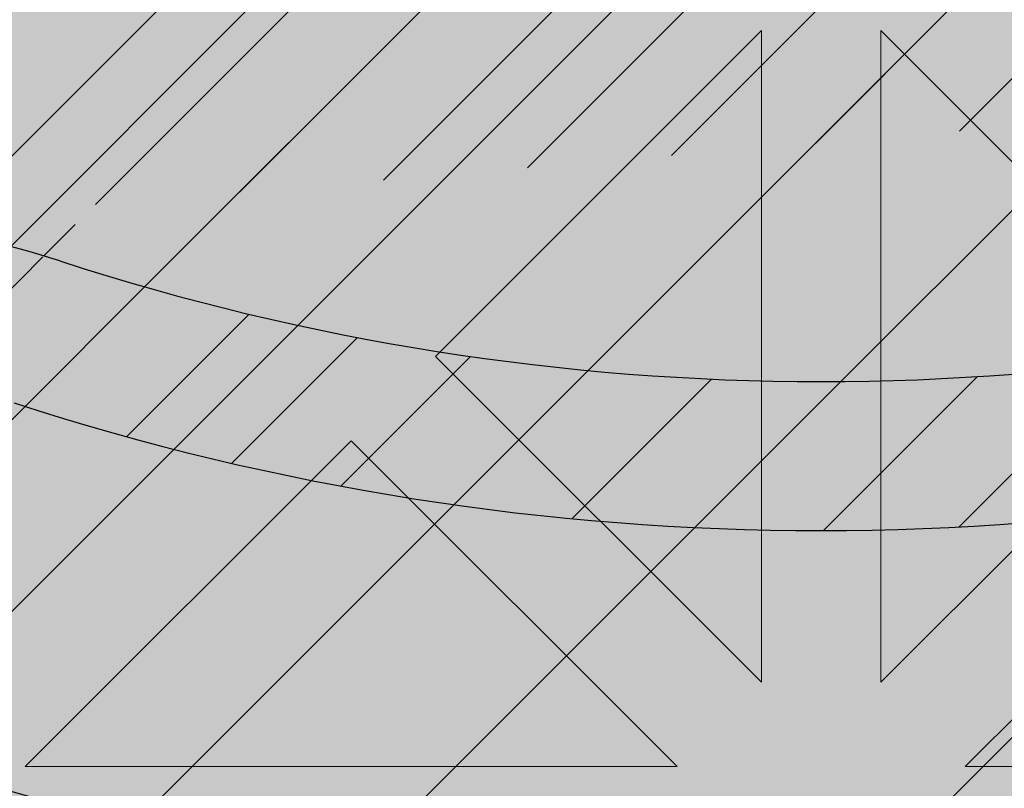
# Model space of a CAD drawing. Units: inches. Extents: x 844 to 2234, y 346 to 1084.
# Tile 10 of 93: x 1121.143 to 1123.249, y 688.619 to 690.263. Entities that reach past the tile are written whole.
import ezdxf

# ---------------------------------------------------------------- set-up
doc = ezdxf.new("R2010")
doc.units = ezdxf.units.IN
doc.header["$MEASUREMENT"] = 0
for name, color, linetype, lineweight in [('A-ANNO-DIMS', 2, 'Continuous', 18), ('furniture', 8, 'Continuous', 18), ('RA-AP-01$0$INT', 35, 'Continuous', 5)]:
    doc.layers.add(name, color=color, linetype=linetype, lineweight=lineweight)
doc.layers.add('RA-AP-01$0$FURN', color=3, linetype='Continuous')
doc.layers.add('RA-AP-01$0$WOOD', color=64, linetype='Continuous')
doc.styles.get("Standard").update_dxf_attribs({"font": 'arial.ttf'})
doc.dimstyles.get("Standard").update_dxf_attribs({"dimtxt": 6, "dimasz": 3, "dimexe": 0.18, "dimexo": 0.0625, "dimgap": 0.09, "dimtad": 0, "dimtih": 1, "dimtoh": 1, "dimdec": 1, "dimzin": 0, "dimdsep": 46, "dimlunit": 3, "dimtxsty": 'Standard', "dimblk": 'ARCHTICK', "dimcen": 0.09, "dimadec": 0, "dimazin": 0, "dimtfac": 1, "dimtdec": 1, "dimtofl": 0, "dimtmove": 0, "dimatfit": 3, "dimfxl": 1, "dimtolj": 1, "dimtzin": 0, "dimarcsym": 0})

# ---------------------------------------------------------------- blocks, each defined once
blk = doc.blocks.new('A$C18D01794')
at = {"layer": 'RA-AP-01$0$INT'}
h = blk.add_hatch(color=256, dxfattribs=at)
h.paths.add_polyline_path([(4.585917135068449, -6.356712009588271), (4.555206456959269, -6.35671200958746), (4.555206456959137, -6.387422687716308), (4.874495778835233, -6.706712009592356), (4.90520645695423, -6.676001331474049)])
h.paths.add_polyline_path([(5.255206456948813, -6.387422687716306), (5.255206456948682, -6.356712009605972), (5.224495778822613, -6.356712009605161), (4.905206456953498, -6.676001331474273), (4.935917135072151, -6.706712009592924)])
h.paths.add_polyline_path([(4.935917135072559, -6.706712009592068), (4.905206456953564, -6.737422687710376), (5.255206456951813, -7.087422687708613), (5.255206456951549, -7.026001331471008)])
h.paths.add_polyline_path([(4.555206456956399, -7.026001331471013), (4.555206456956134, -7.087422687708616), (4.905206456953821, -6.737422687710943), (4.874495778835166, -6.70671200959229)])
h = blk.add_hatch(color=256, dxfattribs=at)
h.paths.add_polyline_path([(4.585917135068448, -6.356712009588273), (4.614201406330596, -6.356712009589021), (4.668846067270487, -6.411356670531338), (4.723490728212344, -6.356712009591912), (4.771774999457151, -6.35671200959319), (4.826419660396886, -6.411356670535356), (4.862780050090322, -6.374996280843536), (4.844495778842715, -6.356712009595112), (4.862780050090411, -6.356712009595595), (4.905206456960182, -6.399138416468211), (4.947632863832445, -6.356712009597838), (4.965917135079675, -6.356712009598322), (4.947632863831759, -6.374996280845421), (4.983993253523576, -6.411356670538857), (5.038637914464627, -6.356712009600247), (5.08692218571208, -6.356712009601523), (5.141566846649976, -6.411356670541852), (5.196211507589851, -6.356712009604411), (5.224495778822615, -6.356712009605161), (4.905206456953975, -6.676001331473793)])
h.paths.add_polyline_path([(4.895206456956031, -6.637717060225675), (4.895206456958921, -6.528427738347902), (4.840561796018589, -6.583072399285802)], flags=16)
h.paths.add_polyline_path([(4.915206456955638, -6.637717060226121), (4.969851117895509, -6.583072399288678), (4.915206456957609, -6.528427738348344)], flags=16)
h.paths.add_polyline_path([(4.826419660395175, -6.568930263661755), (4.881064321335613, -6.514285602723745), (4.771774999456703, -6.514285602720857)], flags=16)
h.paths.add_polyline_path([(4.983993253519558, -6.568930263665262), (5.038637914460456, -6.514285602726792), (4.929348592581548, -6.514285602724816)], flags=16)
h.paths.add_polyline_path([(4.881064321336025, -6.494285602723742), (4.826419660397532, -6.439640941782821), (4.771774999457062, -6.494285602720859)], flags=16)
h.paths.add_polyline_path([(4.929348592582019, -6.494285602724817), (5.038637914460982, -6.494285602726792), (4.983993253522945, -6.439640941786327)], flags=16)
h.paths.add_polyline_path([(4.895206456960191, -6.480143467100443), (4.895206456962115, -6.407422687715913), (4.876922185715016, -6.389138416467584), (4.840561796021581, -6.425498806159401)], flags=16)
h.paths.add_polyline_path([(4.915206456958487, -6.480143467100889), (4.969851117899527, -6.425498806162279), (4.933490728206909, -6.389138416468043), (4.9152064569598, -6.40742268771434)], flags=16)
h.paths.add_polyline_path([(4.757632863832376, -6.480143467096812), (4.812277524772842, -6.425498806158772), (4.757632863834348, -6.370854145217844)], flags=16)
h.paths.add_polyline_path([(4.737632863832376, -6.480143467096286), (4.737632863834348, -6.370854145217375), (4.682988202893906, -6.425498806155385)], flags=16)
h.paths.add_polyline_path([(5.05278005008503, -6.480143467103376), (5.052780050087917, -6.370854145224413), (4.998135389146995, -6.425498806162908)], flags=16)
h.paths.add_polyline_path([(5.072780050085024, -6.480143467103744), (5.127424711025931, -6.42549880616527), (5.072780050087916, -6.370854145224832)], flags=16)
h.paths.add_polyline_path([(4.935917135072783, -6.706712009592292), (5.255206456948811, -6.387422687716309), (5.255206456948932, -6.415706958964177), (5.200561796010279, -6.470351619902839), (5.255206456949403, -6.524996280841948), (5.25520645694961, -6.5732805520894), (5.200561796009787, -6.627925213029239), (5.236922185702417, -6.664285602721864), (5.255206456949919, -6.646001331474357), (5.255206456949998, -6.664285602721898), (5.212780050078687, -6.706712009592262), (5.25520645695036, -6.749138416463932), (5.255206456950438, -6.767422687711313), (5.236922185702424, -6.749138416463297), (5.200561796009796, -6.785498806155928), (5.255206456950753, -6.840143467096874), (5.25520645695096, -6.888427738341682), (5.200561796010322, -6.943072399282328), (5.255206456951428, -6.997717060223427), (5.255206456951547, -7.026001331471006)])
h.paths.add_polyline_path([(5.042988202883395, -6.785498806155427), (5.097632863823085, -6.840143467095101), (5.097632863822622, -6.730854145216193)], flags=16)
h.paths.add_polyline_path([(5.028846067259663, -6.771356670531693), (5.083490728198774, -6.716712009592573), (4.974201406321001, -6.716712009593042)], flags=16)
h.paths.add_polyline_path([(5.117632863823087, -6.840143467095186), (5.172277524762331, -6.785498806155926), (5.11763286382262, -6.730854145216225)], flags=16)
h.paths.add_polyline_path([(5.08349072819877, -6.696712009593886), (5.028846067259652, -6.642067348654775), (4.974201406320998, -6.696712009593438)], flags=16)
h.paths.add_polyline_path([(5.131774999446817, -6.854285602718917), (5.186419660386065, -6.799640941779662), (5.241064321325782, -6.854285602719365)], flags=17)
h.paths.add_polyline_path([(5.131774999446228, -6.716712009592374), (5.186419660386065, -6.771356670532194), (5.222780050079488, -6.734996280838764), (5.204495778832781, -6.716712009592063)], flags=16)
h.paths.add_polyline_path([(5.097632863822613, -6.682569873970264), (5.097632863823061, -6.573280552091354), (5.042988202883383, -6.627925213031044)], flags=16)
h.paths.add_polyline_path([(5.131774999446899, -6.874285602718915), (5.241064321325809, -6.874285602719364), (5.186419660386591, -6.928930263658598)], flags=17)
h.paths.add_polyline_path([(5.131774999446226, -6.696712009594078), (5.204495778830767, -6.696712009594374), (5.22278005007868, -6.67842773834687), (5.186419660386049, -6.642067348654249)], flags=16)
h.paths.add_polyline_path([(5.11763286382262, -6.682569873970225), (5.17227752476232, -6.627925213030515), (5.117632863823064, -6.573280552091267)], flags=16)
h.paths.add_polyline_path([(5.186419660386069, -6.613783077405491), (5.241064321325754, -6.559138416465795), (5.131774999446791, -6.559138416466263)], flags=16)
h.paths.add_polyline_path([(5.131774999446872, -6.539138416466263), (5.24106432132578, -6.539138416465794), (5.186419660386554, -6.484493755526573)], flags=16)
h.paths.add_polyline_path([(5.255206456951811, -7.08742268770861), (5.255206456951895, -7.106712009588038), (4.555206456956052, -7.106712009588038), (4.555206456956136, -7.087422687708617), (4.905206456953973, -6.737422687710788)])
h.paths.add_polyline_path([(4.983993253513404, -6.8444937555241), (4.92934859257295, -6.899138416462108), (5.03863791445186, -6.899138416465014)], flags=16)
h.paths.add_polyline_path([(4.969851117889988, -6.83035161990006), (4.915206456952556, -6.775706958960171), (4.915206456949648, -6.884996280837944)], flags=16)
h.paths.add_polyline_path([(4.929348592572535, -6.919138416462105), (4.983993253511019, -6.973783077403037), (5.038637914451496, -6.919138416465012)], flags=16)
h.paths.add_polyline_path([(5.052780050074912, -6.93328055208906), (4.998135389134438, -6.987925213027088), (5.052780050072919, -7.042569873968025)], flags=16)
h.paths.add_polyline_path([(5.07278005007491, -6.933280552089588), (5.072780050072918, -7.042569873968497), (5.127424711013374, -6.987925213030498)], flags=16)
h.paths.add_polyline_path([(4.89520645695295, -6.775706958959721), (4.840561796013067, -6.830351619897157), (4.895206456950961, -6.884996280837494)], flags=16)
h.paths.add_polyline_path([(4.915206456948365, -6.933280552085403), (4.915206456946434, -7.006001331471951), (4.933490728192729, -7.024285602719066), (4.969851117886972, -6.987925213026453)], flags=16)
h.paths.add_polyline_path([(4.881064321327021, -6.899138416461022), (4.82641966038902, -6.84449375552057), (4.771774999448108, -6.899138416459029)], flags=16)
h.paths.add_polyline_path([(4.895206456950073, -6.933280552084951), (4.840561796009022, -6.987925213023558), (4.876922185700835, -7.024285602716997), (4.895206456948749, -7.006001331469487)], flags=16)
h.paths.add_polyline_path([(4.983993253510392, -7.0020673486505), (4.947632863816944, -7.038427738342319), (4.965917135064043, -7.05671200959023), (5.038637914448995, -7.056712009591555)], flags=16)
h.paths.add_polyline_path([(4.881064321326543, -6.91913841646102), (4.771774999447578, -6.919138416459031), (4.826419660385607, -6.973783077399508)], flags=16)
h.paths.add_polyline_path([(4.905206456946447, -7.014285602717636), (4.862780050074785, -7.056712009588352), (4.947632863816685, -7.056712009589775)], flags=16)
h.paths.add_polyline_path([(5.14156684663679, -7.002067348654549), (5.086922185696452, -7.056712009592438), (5.196211507574223, -7.056712009594425)], flags=16)
h.paths.add_polyline_path([(4.8264196603837, -7.002067348646972), (4.771774999442643, -7.056712009585575), (4.8444957788276, -7.056712009587508), (4.862780050075511, -7.038427738340416)], flags=16)
h.paths.add_polyline_path([(4.812277524760289, -6.98792521302292), (4.757632863822258, -6.933280552082447), (4.757632863819352, -7.042569873961408)], flags=16)
h.paths.add_polyline_path([(4.73763286382226, -6.933280552082079), (4.682988202881349, -6.987925213020536), (4.737632863819352, -7.04256987396099)], flags=16)
h.paths.add_polyline_path([(4.723490728195188, -7.056712009584289), (4.668846067257299, -7.002067348643949), (4.614201406317417, -7.056712009581383)], flags=16)
h.paths.add_polyline_path([(4.597632863829262, -6.706712009592262), (4.555206456957951, -6.664285602721896), (4.555206456958029, -6.646001331474357), (4.573490728205535, -6.664285602721864), (4.609851117898167, -6.627925213029238), (4.555206456958338, -6.573280552089402), (4.555206456958546, -6.524996280841952), (4.60985111789767, -6.470351619902839), (4.555206456959015, -6.415706958964177), (4.555206456959138, -6.387422687716309), (4.874495778835167, -6.70671200959229), (4.5552064569564, -7.026001331471015), (4.555206456956523, -6.997717060223433), (4.609851117897629, -6.94307239928233), (4.555206456956988, -6.888427738341681), (4.555206456957198, -6.840143467096881), (4.609851117898153, -6.78549880615593), (4.573490728205528, -6.749138416463297), (4.555206456957507, -6.76742268771132), (4.555206456957585, -6.749138416463933)])
h.paths.add_polyline_path([(4.712780050085332, -6.730854145216195), (4.712780050084863, -6.840143467095105), (4.767424711024555, -6.785498806155427)], flags=16)
h.paths.add_polyline_path([(4.726922185709173, -6.716712009592573), (4.781566846648288, -6.771356670531693), (4.836211507586949, -6.716712009593043)], flags=16)
h.paths.add_polyline_path([(4.692780050085327, -6.730854145216225), (4.638135389145619, -6.785498806155928), (4.692780050084865, -6.840143467095185)], flags=16)
h.paths.add_polyline_path([(4.726922185709182, -6.696712009593886), (4.836211507586949, -6.696712009593436), (4.7815668466483, -6.642067348654773)], flags=16)
h.paths.add_polyline_path([(4.678637914461726, -6.71671200959237), (4.605917135075169, -6.716712009592063), (4.587632863828464, -6.734996280838766), (4.623993253521887, -6.771356670532195)], flags=16)
h.paths.add_polyline_path([(4.712780050085336, -6.68256987397026), (4.767424711024568, -6.627925213031042), (4.71278005008489, -6.573280552091352)], flags=16)
h.paths.add_polyline_path([(4.678637914461726, -6.696712009594076), (4.623993253521899, -6.642067348654247), (4.587632863829271, -6.67842773834687), (4.605917135077185, -6.696712009594376)], flags=16)
h.paths.add_polyline_path([(4.692780050085336, -6.682569873970228), (4.692780050084889, -6.573280552091267), (4.638135389145632, -6.627925213030515)], flags=16)
h.paths.add_polyline_path([(4.623993253521885, -6.799640941779662), (4.678637914461131, -6.854285602718915), (4.56934859258217, -6.854285602719365)], flags=17)
h.paths.add_polyline_path([(4.623993253521901, -6.613783077405509), (4.678637914461158, -6.559138416466263), (4.569348592582195, -6.559138416465795)], flags=16)
h.paths.add_polyline_path([(4.678637914461051, -6.874285602718915), (4.623993253521361, -6.928930263658598), (4.569348592582143, -6.874285602719364)], flags=17)
h.paths.add_polyline_path([(4.678637914461076, -6.539138416466263), (4.623993253521399, -6.484493755526573), (4.569348592582167, -6.539138416465796)], flags=16)
h = blk.add_hatch(color=256, dxfattribs=at)
h.paths.add_polyline_path([(4.969851117891331, -6.583072399286455), (4.915206456952669, -6.63771706022511), (4.915206456952222, -6.528427738347337)])
h.paths.add_polyline_path([(4.895206456953064, -6.637717060225108), (4.840561796014413, -6.583072399286448), (4.895206456953533, -6.528427738347335)])
h.paths.add_polyline_path([(4.826419660390684, -6.568930263662714), (4.771774999451003, -6.514285602723024), (4.881064321329913, -6.514285602723489)])
h.paths.add_polyline_path([(4.881064321329884, -6.494285602723492), (4.771774999450921, -6.494285602723024), (4.82641966039018, -6.439640941783778)])
h.paths.add_polyline_path([(4.895206456953734, -6.48014346709988), (4.840561796013912, -6.425498806160046), (4.876922185707337, -6.389138416466622), (4.895206456954043, -6.40742268771333)])
h.paths.add_polyline_path([(4.862780050082808, -6.374996280843689), (4.826419660390178, -6.411356670536314), (4.771774999450351, -6.356712009596481), (4.844495778835303, -6.356712009596181)])
h.paths.add_polyline_path([(4.812277524766446, -6.425498806160041), (4.757632863827191, -6.480143467099289), (4.757632863826741, -6.370854145220329)])
h.paths.add_polyline_path([(4.737632863827191, -6.480143467099214), (4.682988202887508, -6.425498806159518), (4.737632863826743, -6.370854145220299)])
h.paths.add_polyline_path([(4.668846067263777, -6.41135667053579), (4.614201406325123, -6.356712009597128), (4.723490728202894, -6.356712009596675)])
h.paths.add_polyline_path([(4.905206456953846, -6.399138416467422), (4.862780050082654, -6.356712009596229), (4.947632863824561, -6.356712009595756)])
h.paths.add_polyline_path([(4.915206456952028, -6.480143467099882), (4.91520645695173, -6.407422687715346), (4.933490728199234, -6.389138416467428), (4.96985111789186, -6.425498806160055)])
h.paths.add_polyline_path([(5.038637914454841, -6.494285602723048), (4.929348592575874, -6.494285602723497), (4.983993253515593, -6.439640941783787)])
h.paths.add_polyline_path([(4.983993253515065, -6.568930263662725), (4.929348592575849, -6.514285602723495), (5.038637914454755, -6.514285602723045)])
h.paths.add_polyline_path([(5.052780050079843, -6.480143467099317), (4.998135389140595, -6.425498806160058), (5.052780050080309, -6.370854145220356)])
h.paths.add_polyline_path([(4.983993253516868, -6.411356670536324), (4.947632863824241, -6.374996280843694), (4.965917135071747, -6.356712009596188), (5.038637914456701, -6.356712009596504)])
h.paths.add_polyline_path([(5.127424711019533, -6.425498806159557), (5.072780050079843, -6.480143467099239), (5.07278005008031, -6.370854145220326)])
h.paths.add_polyline_path([(5.141566846643269, -6.411356670535829), (5.086922185704154, -6.356712009596707), (5.196211507581929, -6.356712009597176)])
for p, q in [((4.905206456953975, -6.676001331473793), (4.585917135071132, -6.356712009590955)), ((4.874495778835167, -6.70671200959229), (4.555206456959136, -6.387422687716307)), ((4.771774999456703, -6.514285602720857), (4.881064321335613, -6.514285602723743)), ((4.826419660395171, -6.568930263661755), (4.771774999456703, -6.514285602720857)), ((4.881064321335613, -6.514285602723743), (4.826419660395173, -6.568930263661757)), ((4.929348592581546, -6.514285602724816), (4.983993253519556, -6.568930263665262)), ((5.038637914460456, -6.514285602726792), (4.929348592581546, -6.514285602724816)), ((4.895206456958917, -6.528427738347906), (4.840561796018589, -6.583072399285802)), ((4.895206456958921, -6.528427738347904), (4.895206456956031, -6.637717060225675)), ((4.915206456957613, -6.52842773834835), (4.969851117895507, -6.583072399288678)), ((4.915206456957609, -6.528427738348348), (4.915206456955636, -6.637717060226119)), ((4.895206456956031, -6.637717060225675), (4.840561796018589, -6.583072399285802)), ((4.915206456955636, -6.637717060226119), (4.969851117895507, -6.583072399288678))]:
    blk.add_line(p, q, dxfattribs=at)
blk = doc.blocks.new('A$C32926AE1')
at = {"layer": 'RA-AP-01$0$FURN'}
h = blk.add_hatch(dxfattribs=at)
h.set_pattern_fill('ANSI31', color=256, scale=0.1, style=0)
h.set_pattern_definition([(45, (0, 0), (-0.0088388347648318, 0.0088388347648318), [])])
edge = h.paths.add_edge_path(flags=16)
edge.add_arc((4.904771284329206, 4.246793130718756), 0.2603971832811541, 75.22398030683196, 104.7760196931204)
edge.add_arc((4.904771284329206, 4.246793130718756), 0.2603971832811541, 75.223980306832, 104.77601969312039, ccw=False)
edge = h.paths.add_edge_path(flags=16)
edge.add_arc((4.904771284329206, 4.067062675376612), 0.2603971832811541, 255.2239803068796, 284.776019693168)
edge.add_arc((4.904771284329206, 4.067062675376612), 0.2603971832811541, 255.22398030687958, 284.77601969316805, ccw=False)
edge = h.paths.add_edge_path(flags=0)
edge.add_arc((4.904771284329206, 4.067062675376612), 0.2603971832811541, 255.2239803068796, 284.776019693168)
edge.add_arc((4.904771284329206, 4.067062675376612), 0.2603971832811541, 255.22398030687958, 284.77601969316805, ccw=False)
edge = h.paths.add_edge_path(flags=0)
edge.add_arc((4.904771284329206, 4.067062675376612), 0.2603971832811541, 255.2239803068796, 284.776019693168)
edge.add_arc((4.904771284329206, 4.067062675376612), 0.2603971832811541, 255.22398030687958, 284.77601969316805, ccw=False)
edge = h.paths.add_edge_path()
edge.add_arc((4.604388392048174, 4.588829985554312), 0.1599999999999918, 342.3781640246255, 354.4317409793762)
edge.add_arc((5.090145208887507, 4.43216705527679), 0.3503971832811637, 162.0091218307731, 180.3186872093483)
edge.add_arc((5.205154176610243, 4.588829985554953), 0.1599999999999917, 185.5682590208461, 197.6218359767349)
edge.add_arc((4.904771284329229, 4.246793130718735), 0.3503971832811761, 72.00912183053516, 107.9908781690354)
edge.add_arc((9.535952835716557, 4.28682295566602), 4.798342501046485, 178.2875002453811, 181.5576802719453)
edge.add_arc((4.719397359771122, 4.43216705527679), 0.3503971832811637, 359.6813127906516, 377.9908781692269)
edge.add_arc((9.535967292294904, 4.286822350292874), 4.778371420254705, 178.2965938931842, 181.5667745797229)
edge.add_arc((4.719397359771122, 4.43216705527679), 0.3303971832811637, 359.6813127906516, 377.9908781692269)
edge.add_arc((0.2735752763637294, 4.286822350292874), 4.7783714202547, 358.4332254202771, 361.7034061068158)
edge.add_arc((5.061434214606998, 4.732549947558029), 0.1600000000000254, 252.3781640250584, 264.4317409792362)
edge.add_arc((4.748108354051257, 4.732549947558012), 0.1600000000000541, 275.5682590208426, 287.6218359759532)
edge.add_arc((4.604388392048115, 4.588829985554317), 0.1800000000000505, 342.3567572500182, 349.3735009646207)
edge.add_arc((5.205154176610254, 4.588829985554976), 0.1800000000000069, 190.6264990356027, 197.6432427513933)
edge.add_arc((5.061434214607106, 4.732549947558013), 0.1800000000000424, 252.3567572496606, 259.3735009644582)
edge.add_arc((4.904771284329208, 4.246793130718737), 0.3303971832811676, 71.99844483668534, 108.0015551637021)
edge.add_arc((4.748108354051414, 4.732549947558045), 0.1800000000000547, 280.6264990355479, 287.6432427495938)
edge.add_arc((5.090145208887514, 4.432167055276789), 0.2803971832811691, 162.8706300666893, 180.816523289902)
edge.add_arc((4.719397359771136, 4.432167055276689), 0.2803971832811534, 359.183476710103, 377.1293699333214)
edge.add_arc((4.904771284329222, 4.246793130718737), 0.2803971832811769, 72.87063006672916, 107.1293699332334)
edge.add_arc((5.090145208887522, 4.432167055276788), 0.2603971832811776, 165.2239803068007, 180.9953123810312)
edge.add_arc((4.719397359771141, 4.432167055276699), 0.2603971832811458, 359.0046876189768, 374.7760196932087)
edge.add_arc((5.090145208887507, 4.43216705527679), 0.3303971832811637, 162.0091218307731, 180.3186872093483)
edge.add_arc((9.53595427642584, 4.285015535491528), 4.728345371032053, 178.265043920078, 181.5679956281801)
edge.add_arc((0.2735882922327999, 4.285015535491582), 4.728345371032045, 358.4320043718193, 361.7349560799204)
edge.add_arc((9.535953591267507, 4.284458026472751), 4.708343996644348, 178.2573054306777, 181.5704995759608)
edge.add_arc((0.273588977391114, 4.284458026472785), 4.708343996644358, 358.4295004240388, 361.7426945693213)
edge.add_arc((0.2735889773911131, 4.029397779622582), 4.708343996644359, 358.2573054306787, 361.5704995759613)
edge.add_arc((9.535953591267518, 4.029397779622618), 4.708343996644359, 178.4295004240391, 181.7426945693223)
edge.add_arc((0.2735882922327901, 4.028840270603786), 4.728345371032054, 358.2650439200796, 361.5679956281808)
edge.add_arc((9.53595427642584, 4.028840270603841), 4.728345371032054, 178.4320043718199, 181.7349560799219)
edge.add_arc((0.2735752763637302, 4.027033455802493), 4.778371420254699, 358.2965938931842, 361.5667745797229)
edge.add_arc((4.719397359771122, 3.881688750818578), 0.3303971832811637, 342.0091218307731, 360.3186872093484)
edge.add_arc((5.090145208887507, 3.881688750818578), 0.3303971832811637, 179.6813127906516, 197.9908781692269)
edge.add_arc((9.535967292294904, 4.027033455802493), 4.778371420254705, 178.433225420277, 181.7034061068158)
edge.add_arc((4.719397359771122, 3.881688750818578), 0.3503971832811637, 342.0091218307731, 360.3186872093484)
edge.add_arc((9.53595283571655, 4.027032850429349), 4.79834250104648, 178.4423197280546, 181.7124997546188)
edge.add_arc((4.719397359771141, 3.881688750818669), 0.2603971832811458, 345.2239803067913, 360.9953123810232)
edge.add_arc((5.090145208887522, 3.88168875081858), 0.2603971832811776, 179.0046876189687, 194.7760196931993)
edge.add_arc((4.904771284329222, 4.067062675376631), 0.2803971832811769, 252.8706300667665, 287.1293699332708)
edge.add_arc((4.719397359771136, 3.881688750818678), 0.2803971832811534, 342.8706300666787, 360.8165232898969)
edge.add_arc((5.090145208887514, 3.881688750818579), 0.2803971832811691, 179.183476710098, 197.1293699333106)
edge.add_arc((4.748108354051414, 3.581305858537323), 0.1800000000000547, 72.3567572504062, 79.37350096445199)
edge.add_arc((4.904771284329208, 4.067062675376631), 0.3303971832811676, 251.9984448362979, 288.0015551633146)
edge.add_arc((5.061434214607106, 3.581305858537355), 0.1800000000000424, 100.6264990355418, 107.6432427503394)
edge.add_arc((5.205154176610254, 3.725025820540392), 0.1800000000000069, 162.3567572486066, 169.3735009643972)
edge.add_arc((4.604388392048115, 3.725025820541051), 0.1800000000000505, 10.62649903537925, 17.64324274998182)
edge.add_arc((4.748108354051257, 3.581305858537356), 0.1600000000000541, 72.37816402404681, 84.43174097915735)
edge.add_arc((4.904771284329229, 4.067062675376632), 0.3503971832811761, 252.0091218309645, 287.9908781694648)
edge.add_arc((5.061434214606998, 3.581305858537339), 0.1600000000000254, 95.56825902076373, 107.6218359749416)
edge.add_arc((5.205154176610243, 3.725025820540414), 0.1599999999999917, 162.3781640232651, 174.4317409791539)
edge.add_arc((5.090145208887507, 3.881688750818578), 0.3503971832811637, 179.6813127906516, 197.9908781692269)
edge.add_arc((4.604388392048174, 3.725025820541056), 0.1599999999999918, 5.568259020623824, 17.62183597537444)
edge.add_arc((0.2735897329420762, 4.28682295566602), 4.798342501046482, 358.4423197280547, 361.7124997546188)
edge.add_arc((0.2735897329420691, 4.027032850429348), 4.798342501046489, 358.2875002453812, 361.5576802719453)
at = {"layer": 'RA-AP-01$0$WOOD'}
h = blk.add_hatch(color=256, dxfattribs=at)
h.dxf.hatch_style = 1
h.paths.add_polyline_path([(5.157430609644524, 4.573483066760929, -0.1009492694046607), (5.155401577623758, 4.593365984175333, -0.1842662638101597), (5.172249623284174, 4.638795604568598, 0.2056608120311276), (5.179560981299304, 4.661316324430096, 0.3614336704623542), (5.134352340494423, 4.706524965234944, 0.2056608120311297), (5.111831620632933, 4.699213607219793, -0.1842662638101113), (5.066402000239693, 4.682365561559342, -0.1055311479399994), (5.045656153913092, 4.68467289944697, 0.1567636581983829), (4.763886414745334, 4.684672899446966, -0.1055311479399895), (4.743140568418733, 4.68236556155934, -0.1842662638100833), (4.6977109480255, 4.69921360721979, 0.2056608120302612), (4.675190228164109, 4.706524965234949, 0.3614336704708441), (4.629981587358889, 4.66131632442871, 0.2056608120245944), (4.637292945374126, 4.638795604567974, -0.1842662638101024), (4.654140991034615, 4.59336598417475, -0.1009492694055169), (4.652111959013835, 4.573483066760181, 0.021410119221476), (4.629748025606143, 4.156712009541676, 0.0214101192214795), (4.652111959013809, 3.739940952323101, -0.1009492694059586), (4.654140991034615, 3.720058034908448, -0.1842662638100975), (4.637292945374126, 3.674628414515226, 0.2056608120245705), (4.629981587358889, 3.652107694654492, 0.3614336704708879), (4.675190228164113, 3.606899053848249, 0.2056608120302384), (4.697710948025501, 3.614210411863408, -0.1842662638100995), (4.743140568418738, 3.63105845752386, -0.1055311479402541), (4.763886414745388, 3.628751119636215, 0.1567636581983776), (5.045656153913137, 3.628751119636244, -0.1055311479397538), (5.066402000239692, 3.631058457523857, -0.1842662638101067), (5.111831620632931, 3.614210411863407, 0.2056608120310924), (5.134352340494417, 3.606899053848256, 0.3614336704624001), (5.179560981299307, 3.652107694653103, 0.2056608120311314), (5.172249623284175, 3.6746284145146, -0.1842662638101402), (5.155401577623758, 3.72005803490786, -0.1009492694051366), (5.15743060964455, 3.739940952322354, 0.0214101192215073), (5.179794543052287, 4.156712009541468, 0.0214101192215252)])
h.paths.add_polyline_path([(4.639748609479751, 4.156712009541513, 0.0213537860821624), (4.661970494867118, 3.741887061152232, -0.094075836301374), (4.664143710413708, 3.7196126951003, -0.1824818158568985), (4.644813765429836, 3.668037719127816, 0.2056608120245319), (4.639939526753007, 3.653023905887301, 0.3614336704710246), (4.676106439397173, 3.616856993242342, 0.2056608120302234), (4.691120252638095, 3.621731231919122, -0.1824818158602558), (4.742695228611606, 3.641061176902986, -0.1029891339458722), (4.766991894714349, 3.638256818950944, 0.156709409989566), (5.042550673941472, 3.638256818950105, -0.102989133958497), (5.066847340047078, 3.641061176902949, -0.1824818158594995), (5.118422316020358, 3.621731231919103, 0.2056608120311416), (5.133436129261316, 3.616856993242346, 0.3614336704621468), (5.169603041905217, 3.653023905886178, 0.2056608120310986), (5.164728803228477, 3.668037719127177, -0.1824818158565612), (5.145398858244737, 3.719612695099578, -0.0940758363009313), (5.147572073791232, 3.741887061151398, 0.0213537860822023), (5.169793959178681, 4.156712009541451, 0.0213537860822226), (5.147572073791203, 4.571536957931898, -0.0940758363005034), (5.145398858244737, 4.59381132398362, -0.1824818158565587), (5.164728803228476, 4.645386299956021, 0.2056608120311045), (5.169603041905216, 4.66040011319702, 0.3614336704621845), (5.133436129261313, 4.696567025840856, 0.2056608120310773), (5.118422316020359, 4.691692787164098, -0.182481815859508), (5.066847340047078, 4.67236284218025, -0.1029891339584606), (5.04255067394148, 4.675167200133092, 0.156709409989566), (4.766991894714357, 4.675167200132257, -0.1029891339458842), (4.742695228611611, 4.672362842180213, -0.1824818158602725), (4.691120252638095, 4.691692787164077, 0.2056608120302152), (4.676106439397174, 4.696567025840858, 0.3614336704710363), (4.639939526753005, 4.660400113195899, 0.2056608120245495), (4.644813765429837, 4.645386299955384, -0.1824818158568934), (4.664143710413708, 4.593811323982902, -0.0940758363009187), (4.661970494867149, 4.571536957931074, 0.021353786082177)], flags=16)
h.paths.add_polyline_path([(5.129794543052235, 4.432167055276933, -0.0141661062790638), (5.130152669293814, 4.156927903047693, -0.0141661062790647), (5.129794543052234, 3.881688750818433, -0.0785247771143638), (5.10979738006795, 3.755143611847103, 0.0945969212073497), (5.105408519571111, 3.717898134952927, 0.1043170707844957), (5.116074640131521, 3.670385395016088, 0.1043170707864965), (5.068561900193738, 3.681051515576561, 0.09459692119553), (5.031316423304057, 3.676662655080835, -0.1580239521427272), (4.778226145355827, 3.676662655080367, 0.0945969211986668), (4.740980668464973, 3.681051515576592, 0.1043170707882822), (4.693467928526415, 3.670385395015844, 0.1043170707867916), (4.704134049087309, 3.717898134953662, 0.0945969211972894), (4.69974518859162, 3.755143611844042, -0.0785247771163196), (4.679748025606343, 3.881688750818406, -0.0141661062790663), (4.679389899364763, 4.156927903047693, -0.0141661062790672), (4.679748025606343, 4.432167055276998, -0.0785247771163064), (4.699745188591625, 4.55871219425134, 0.094596921197333), (4.704134049087308, 4.595957671141738, 0.1043170707867205), (4.693467928526416, 4.643470411079523, 0.1043170707882628), (4.740980668464965, 4.632804290518776, 0.0945969211988114), (4.778226145355874, 4.637193151015016, -0.158023952142669), (5.031316423304015, 4.637193151014546, 0.0945969211956361), (5.068561900193736, 4.632804290518806, 0.1043170707864979), (5.11607464013152, 4.643470411079278, 0.1043170707844617), (5.105408519571112, 4.595957671142455, 0.0945969212074597), (5.109797380067959, 4.558712194248236, -0.0785247771143467)], flags=0)
h.paths.add_polyline_path([(5.119794532311105, 4.432259799204851, -0.0142000800617244), (5.120156169157484, 4.156927903047701, -0.0142000800617277), (5.119794532311105, 3.881596006890482, -0.0784894509520253), (5.100273383573699, 3.758192358677797, 0.0940138827242913), (5.095413455884425, 3.717477693979438, 0.0606271852308753), (5.099615656341024, 3.686844378806616, 0.0606271852322524), (5.068982341167493, 3.691046579263239, 0.0940138827010453), (5.028267676478798, 3.686186651576848, -0.1580706864508061), (4.781274892180912, 3.686186651576435, 0.0940138827026903), (4.740560227491556, 3.691046579263279, 0.0606271852339895), (4.709926912317155, 3.686844378806508, 0.0606271852329405), (4.714129112773991, 3.717477693980356, 0.094013882701304), (4.709269185087677, 3.758192358669163, -0.0784894509577193), (4.689748036347473, 3.881596006890469, -0.014200080061729), (4.689386399501094, 4.156927903047709, -0.0142000800617217), (4.689748036347473, 4.432259799204808, -0.078489450957724), (4.709269185087651, 4.555663447426125, 0.0940138827014585), (4.714129112773992, 4.596378112114996, 0.0606271852329731), (4.709926912317154, 4.62701142728886, 0.0606271852340196), (4.74056022749157, 4.622809226832087, 0.0940138827024997), (4.781274892180847, 4.627669154518912, -0.1580706864508359), (5.028267676478777, 4.627669154518526, 0.0940138827010946), (5.068982341167492, 4.622809226832129, 0.060627185232254), (5.099615656341024, 4.627011427288751, 0.0606271852308727), (5.095413455884425, 4.59637811211593, 0.0940138827241088), (5.100273383573675, 4.555663447417647, -0.0784894509520978)], flags=0)
h.paths.add_polyline_path([(5.06978912287499, 4.430218106756144, -0.014241683694547), (5.070173729147532, 4.156927903047672, -0.0142416836945458), (5.06978912287499, 3.883637699339223, -0.0800609523125196), (5.052662118612511, 3.773463122773442, 0.0526421978001116), (5.04590916754064, 3.740550867606997, 0.0526421977992423), (5.012996912374707, 3.73379791653534, -0.1583028414718258), (4.796545656286308, 3.73379791653451, 0.0526421978034211), (4.763633401117837, 3.740550867607021, 0.0526421978018622), (4.756880450045755, 3.773463122774558, -0.0800609523117106), (4.739753445783639, 3.883637699339268, -0.0142416836945435), (4.739368839511098, 4.156927903047671, -0.0142416836945477), (4.739753445783639, 4.430218106756155, -0.0800609523116345), (4.75688045004574, 4.540392683320762, 0.052642197801941), (4.763633401117837, 4.573304938488346, 0.0526421978035071), (4.796545656286361, 4.580057889560873, -0.1583028414717561), (5.012996912374669, 4.580057889560039, 0.0526421977993048), (5.04590916754064, 4.57330493848837, 0.0526421978002057), (5.052662118612529, 4.540392683321868, -0.080060952312477)], flags=0)
h.paths.add_polyline_path([(5.049789715110557, 4.43038092723357, -0.0143097550741839), (5.05018085590259, 4.156927903047715, -0.0143097550741854), (5.049789715110558, 3.883474878861827, -0.0800685599149176), (5.03362098255317, 3.779581877367999, 0.0306258898956367), (5.028241146483733, 3.758218888663947, 0.0306258898977031), (5.006878157778253, 3.75283905259408, -0.1583983521624096), (4.802664410878162, 3.752839052594731, 0.0306258898946014), (4.781301422174808, 3.758218888663924, 0.0306258898967912), (4.775921586105202, 3.779581877368794, -0.080068559914251), (4.759752853548071, 3.883474878861786, -0.0143097550741854), (4.759361712756037, 4.156927903047671, -0.0143097550741854), (4.759752853548071, 4.430380927233557, -0.0800685599142479), (4.775921586105193, 4.534273928726546, 0.0306258898968306), (4.781301422174808, 4.555636917431444, 0.0306258898945754), (4.802664410878143, 4.561016753500631, -0.1583983521624168), (5.006878157778244, 4.561016753501291, 0.0306258898977177), (5.028241146483733, 4.555636917431421, 0.0306258898958182), (5.03362098255321, 4.534273928727244, -0.080068559914796)], flags=0)
h.paths.add_polyline_path([(4.999766070382627, 4.428171244713864, -0.0143443147609634), (5.000198441819402, 4.156927903047689, -0.0143443147609612), (4.999766070382627, 3.885684561381556, -0.0784641635803329), (4.987356730658798, 3.799103304488872, -0.1506053783831347), (4.822185837999821, 3.79910330448882, -0.0784641635803318), (4.809776498276007, 3.885684561381509, -0.014344314760963), (4.809344126839227, 4.156927903047677, -0.0143443147609645), (4.809776498276007, 4.428171244713873, -0.0784641635803192), (4.822185837999822, 4.514752501606549, -0.1506053783831338), (4.987356730658798, 4.514752501606494, -0.078464163580285)], flags=0)
h.paths.add_polyline_path([(4.979755254238824, 4.42764379880488, -0.0143772539198268), (4.980205517789977, 4.156927903047693, -0.0143772539198275), (4.979755254238824, 3.886212007290489, -0.0689242507424422), (4.971183264704897, 3.815276770442801, -0.1296645318904179), (4.838359303953726, 3.815276770442746, -0.0689242507424186), (4.829787314419809, 3.886212007290419, -0.0143772539198292), (4.829337050868653, 4.156927903047653, -0.0143772539198325), (4.829787314419809, 4.427643798804946, -0.0689242507424211), (4.838359303953725, 4.498579035652621, -0.1296645318904187), (4.971183264704897, 4.498579035652565, -0.0689242507424401)], flags=0)
h = blk.add_hatch(color=256, dxfattribs=at)
h.dxf.hatch_style = 1
h.paths.add_polyline_path([(5.145398858244737, 4.59381132398362, -0.1824818158565616), (5.164728803228476, 4.645386299956021, 0.2056608120311045), (5.169603041905216, 4.66040011319702, 0.3614336704621845), (5.133436129261313, 4.696567025840856, 0.2056608120310773), (5.118422316020359, 4.691692787164098, -0.182481815859508), (5.066847340047078, 4.67236284218025, -0.1029891339584606), (5.04255067394148, 4.675167200133092, 0.156709409989566), (4.766991894714357, 4.675167200132257, -0.1029891339458842), (4.742695228611611, 4.672362842180213, -0.1824818158602725), (4.691120252638095, 4.691692787164077, 0.2056608120302152), (4.676106439397174, 4.696567025840858, 0.3614336704710363), (4.639939526753005, 4.660400113195899, 0.2056608120245495), (4.644813765429837, 4.645386299955384, -0.1824818158568934), (4.664143710413708, 4.593811323982902, -0.0940758363009187), (4.661970494867149, 4.571536957931074, 0.0213537860821772), (4.639748609479751, 4.156712009541507, 0.0213537860821625), (4.661970494867119, 3.741887061152226, -0.0940758363013071), (4.664143710413708, 3.719612695100309, -0.1824818158569294), (4.644813765429836, 3.668037719127816, 0.2056608120245319), (4.639939526753007, 3.653023905887301, 0.3614336704710246), (4.676106439397173, 3.616856993242342, 0.2056608120302234), (4.691120252638095, 3.621731231919122, -0.1824818158602558), (4.742695228611606, 3.641061176902986, -0.1029891339458722), (4.766991894714349, 3.638256818950944, 0.156709409989566), (5.042550673941472, 3.638256818950105, -0.102989133958497), (5.066847340047078, 3.641061176902949, -0.1824818158594995), (5.118422316020358, 3.621731231919103, 0.2056608120311416), (5.133436129261316, 3.616856993242346, 0.3614336704621468), (5.169603041905217, 3.653023905886178, 0.2056608120310986), (5.164728803228477, 3.668037719127177, -0.1824818158565612), (5.145398858244737, 3.719612695099578, -0.0940758363009313), (5.147572073791232, 3.741887061151398, 0.0213537860822023), (5.169793959178681, 4.156712009541451, 0.0213537860822226), (5.147572073791203, 4.571536957931898, -0.0940758363004996)])
h.paths.add_polyline_path([(5.109797380067958, 4.55871219424824, -0.0785247771143472), (5.129794543052234, 4.432167055276936, -0.0141661062790644), (5.130152669293814, 4.156927903047685, -0.014166106279066), (5.129794543052234, 3.881688750818401, -0.0785247771143517), (5.109797380067946, 3.755143611847092, 0.0945969212073132), (5.105408519571111, 3.717898134952929, 0.1043170707844995), (5.116074640131521, 3.670385395016088, 0.1043170707864965), (5.068561900193738, 3.681051515576561, 0.09459692119553), (5.031316423304057, 3.676662655080835, -0.1580239521427272), (4.778226145355827, 3.676662655080367, 0.0945969211986668), (4.740980668464973, 3.681051515576592, 0.1043170707882822), (4.693467928526415, 3.670385395015844, 0.1043170707867916), (4.704134049087309, 3.717898134953662, 0.0945969211972894), (4.69974518859162, 3.755143611844042, -0.0785247771163196), (4.679748025606343, 3.881688750818406, -0.0141661062790663), (4.679389899364763, 4.156927903047693, -0.0141661062790672), (4.679748025606343, 4.432167055276998, -0.0785247771163064), (4.699745188591625, 4.55871219425134, 0.094596921197333), (4.704134049087308, 4.595957671141738, 0.1043170707867205), (4.693467928526416, 4.643470411079523, 0.1043170707882628), (4.740980668464965, 4.632804290518776, 0.0945969211988114), (4.778226145355874, 4.637193151015016, -0.158023952142669), (5.031316423304015, 4.637193151014546, 0.0945969211956361), (5.068561900193736, 4.632804290518806, 0.1043170707864979), (5.11607464013152, 4.643470411079278, 0.1043170707844617), (5.105408519571112, 4.595957671142455, 0.0945969212074504)], flags=16)
h.paths.add_polyline_path([(5.100273383573655, 4.55566344741771, -0.0784894509521388), (5.119794532311105, 4.432259799204852, -0.0142000800617252), (5.120156169157484, 4.156927903047686, -0.014200080061726), (5.119794532311105, 3.881596006890502, -0.0784894509520446), (5.100273383573696, 3.758192358677786, 0.0940138827242721), (5.095413455884425, 3.717477693979436, 0.0606271852308692), (5.099615656341024, 3.686844378806616, 0.0606271852322522), (5.068982341167493, 3.691046579263239, 0.0940138827010453), (5.028267676478798, 3.686186651576848, -0.1580706864508061), (4.781274892180912, 3.686186651576435, 0.0940138827026903), (4.740560227491556, 3.691046579263279, 0.0606271852339895), (4.709926912317155, 3.686844378806508, 0.0606271852329405), (4.714129112773991, 3.717477693980356, 0.094013882701304), (4.709269185087677, 3.758192358669163, -0.0784894509577193), (4.689748036347473, 3.881596006890469, -0.014200080061729), (4.689386399501094, 4.156927903047709, -0.0142000800617217), (4.689748036347473, 4.432259799204808, -0.078489450957724), (4.709269185087651, 4.555663447426125, 0.0940138827014585), (4.714129112773992, 4.596378112114996, 0.0606271852329731), (4.709926912317154, 4.62701142728886, 0.0606271852340196), (4.74056022749157, 4.622809226832087, 0.0940138827024997), (4.781274892180847, 4.627669154518912, -0.1580706864508359), (5.028267676478777, 4.627669154518526, 0.0940138827010946), (5.068982341167492, 4.622809226832129, 0.060627185232254), (5.099615656341024, 4.627011427288751, 0.0606271852308727), (5.095413455884425, 4.59637811211593, 0.094013882723957)], flags=0)
h.paths.add_polyline_path([(5.04590916754064, 4.57330493848837, 0.0526421978002057), (5.052662118612529, 4.540392683321868, -0.0800609523124783), (5.06978912287499, 4.430218106756142, -0.0142416836945469), (5.070173729147532, 4.156927903047672, -0.0142416836945458), (5.06978912287499, 3.883637699339223, -0.0800609523125196), (5.052662118612511, 3.773463122773442, 0.0526421978001116), (5.04590916754064, 3.740550867606997, 0.0526421977992423), (5.012996912374707, 3.73379791653534, -0.1583028414718258), (4.796545656286308, 3.73379791653451, 0.0526421978034211), (4.763633401117837, 3.740550867607021, 0.0526421978018622), (4.756880450045755, 3.773463122774558, -0.0800609523117106), (4.739753445783639, 3.883637699339268, -0.0142416836945435), (4.739368839511098, 4.156927903047671, -0.0142416836945477), (4.739753445783639, 4.430218106756155, -0.0800609523116345), (4.75688045004574, 4.540392683320762, 0.052642197801941), (4.763633401117837, 4.573304938488346, 0.0526421978035071), (4.796545656286361, 4.580057889560873, -0.1583028414717561), (5.012996912374669, 4.580057889560039, 0.0526421977993048)], flags=0)
h.paths.add_polyline_path([(5.028241146483733, 4.555636917431422, 0.0306258898956949), (5.033620982553182, 4.534273928727329, -0.0800685599148649), (5.049789715110557, 4.430380927233569, -0.0143097550741839), (5.05018085590259, 4.156927903047715, -0.0143097550741854), (5.049789715110558, 3.883474878861827, -0.0800685599149176), (5.03362098255317, 3.779581877367999, 0.0306258898956367), (5.028241146483733, 3.758218888663947, 0.0306258898977031), (5.006878157778253, 3.75283905259408, -0.1583983521624096), (4.802664410878162, 3.752839052594731, 0.0306258898946014), (4.781301422174808, 3.758218888663924, 0.0306258898967912), (4.775921586105202, 3.779581877368794, -0.080068559914251), (4.759752853548071, 3.883474878861786, -0.0143097550741854), (4.759361712756037, 4.156927903047671, -0.0143097550741854), (4.759752853548071, 4.430380927233557, -0.0800685599142479), (4.775921586105193, 4.534273928726546, 0.0306258898968306), (4.781301422174808, 4.555636917431444, 0.0306258898945754), (4.802664410878143, 4.561016753500631, -0.1583983521624168), (5.006878157778244, 4.561016753501291, 0.0306258898977174)], flags=0)
h.paths.add_polyline_path([(4.987356730658798, 4.514752501606494, -0.0784641635803018), (4.999766070382627, 4.428171244713845, -0.0143443147609637), (5.000198441819402, 4.156927903047665, -0.0143443147609622), (4.999766070382628, 3.885684561381514, -0.0784641635802952), (4.987356730658797, 3.799103304488872, -0.1506053783831338), (4.822185837999821, 3.799103304488819, -0.0784641635803342), (4.809776498276007, 3.885684561381512, -0.0143443147609628), (4.809344126839227, 4.156927903047676, -0.0143443147609646), (4.809776498276007, 4.428171244713873, -0.0784641635803192), (4.822185837999822, 4.514752501606549, -0.1506053783831338)], flags=0)
h.paths.add_polyline_path([(4.971183264704897, 4.498579035652566, -0.0689242507424384), (4.979755254238824, 4.427643798804883, -0.0143772539198276), (4.980205517789977, 4.15692790304768, -0.0143772539198258), (4.979755254238823, 3.88621200729051, -0.0689242507424628), (4.971183264704897, 3.815276770442801, -0.129664531890417), (4.838359303953726, 3.815276770442746, -0.0689242507424186), (4.829787314419809, 3.886212007290419, -0.0143772539198292), (4.829337050868653, 4.156927903047653, -0.0143772539198325), (4.829787314419809, 4.427643798804946, -0.0689242507424211), (4.838359303953725, 4.498579035652621, -0.1296645318904187)], flags=0)
h = blk.add_hatch(dxfattribs=at)
h.set_pattern_fill('ANSI31', color=256, scale=0.05, style=0)
h.set_pattern_definition([(45, (0, 0), (-0.0044194173824159, 0.0044194173824159), [])])
h.paths.add_polyline_path([(5.130152669293814, 4.156927903047704, 0.0141661062790657), (5.129794543052234, 4.432167055276982, 0.0777827904001433), (5.110168979996553, 4.557559993161921, -0.0976515123401879), (5.105408519571111, 4.595957671142454, -0.1043170707844687), (5.116074640131522, 4.64347041107928), (5.099615656341024, 4.627011427288751, 0.0606271852308727), (5.095413455884425, 4.59637811211593, 0.0940138827241088), (5.100273383573675, 4.555663447417647, -0.0784894509520972), (5.119794532311105, 4.432259799204852, -0.0142000800617252), (5.120156169157484, 4.156927903047686, -0.014200080061726), (5.119794532311105, 3.881596006890502, -0.0784894509520446), (5.100273383573696, 3.758192358677786, 0.0940138827242721), (5.095413455884425, 3.717477693979436, 0.0606271852308692), (5.099615656341024, 3.686844378806616), (5.116074640131519, 3.67038539501609, -0.1043170707844594), (5.105408519571112, 3.717898134952912, -0.0976515123401594), (5.11016897999655, 3.756295812933435, 0.0777827904001654), (5.129794543052234, 3.881688750818409, 0.0141661062790665)])
h.paths.add_polyline_path([(5.030164222210597, 3.676291055149937, -0.0976515123472002), (5.068561900193739, 3.681051515576561, -0.1043170707864927), (5.116074640131521, 3.670385395016088), (5.099615656341024, 3.686844378806616, 0.0606271852322522), (5.068982341167493, 3.691046579263239, 0.0940138827010453), (5.028267676478798, 3.686186651576848, -0.1580706864508061), (4.781274892180912, 3.686186651576435, 0.0940138827026903), (4.740560227491556, 3.691046579263279, 0.0606271852339913), (4.709926912317154, 3.686844378806508), (4.693467928526416, 3.670385395015845, -0.1043170707882796), (4.740980668464973, 3.681051515576592, -0.0976515123427246), (4.779378346446416, 3.676291055150394, 0.156512506893803)])
h.paths.add_polyline_path([(4.689748036347473, 3.881596006890472, -0.014200080061729), (4.689386399501094, 4.156927903047712, -0.0142000800617195), (4.689748036347473, 4.432259799204768, -0.078489450957742), (4.709269185087648, 4.555663447426114, 0.0940138827014821), (4.714129112773992, 4.596378112114995, 0.0606271852329748), (4.709926912317154, 4.62701142728886), (4.693467928526414, 4.643470411079524, -0.1043170707867939), (4.704134049087309, 4.595957671141706, -0.09765151234893), (4.699373588660725, 4.557559993157876, 0.0777827903975372), (4.679748025606343, 4.432167055276987, 0.0141661062790675), (4.679389899364763, 4.156927903047675, 0.0141661062790641), (4.679748025606343, 3.88168875081843, 0.0777827903975637), (4.699373588660724, 3.756295812937497, -0.0976515123490278), (4.704134049087308, 3.717898134953629, -0.1043170707867196), (4.693467928526416, 3.670385395015845), (4.709926912317155, 3.686844378806508, 0.0606271852329413), (4.714129112773991, 3.717477693980357, 0.0940138827013084), (4.709269185087676, 3.758192358669166, -0.0784894509577192)])
h.paths.add_polyline_path([(4.779378346446434, 4.63756475094498, -0.0976515123427943), (4.740980668464964, 4.632804290518776, -0.1043170707882609), (4.693467928526416, 4.643470411079523), (4.709926912317154, 4.62701142728886, 0.0606271852340196), (4.74056022749157, 4.622809226832087, 0.0940138827024997), (4.781274892180847, 4.627669154518912, -0.1580706864508359), (5.028267676478777, 4.627669154518526, 0.0940138827010946), (5.068982341167492, 4.622809226832129, 0.060627185232254), (5.099615656341024, 4.627011427288751), (5.116074640131521, 4.643470411079279, -0.1043170707865022), (5.068561900193735, 4.632804290518806, -0.0976515123475899), (5.030164222210446, 4.637564750945479, 0.1565125068936924)])
h = blk.add_hatch(dxfattribs=at)
h.set_pattern_fill('ANSI32', color=256, scale=0.2, style=0)
h.set_pattern_definition([(45, (0, 0), (-0.0530330085889911, 0.0530330085889911), []), (45, (0.035355339, 0), (-0.0530330085889911, 0.0530330085889911), [])])
h.paths.add_polyline_path([(5.119794532311105, 4.432259799204823, 0.0777015974868765), (5.10065834347252, 4.554469821747928, -0.0968902511992216), (5.095413455884425, 4.596378112115931, -0.060627185230871), (5.099615656341024, 4.627011427288751, -0.060627185232254), (5.068982341167492, 4.622809226832129, -0.0968902512198245), (5.027074050790956, 4.628054114423209, 0.1564657949319105), (4.782468517866163, 4.628054114422785, -0.0968902512152247), (4.740560227491555, 4.622809226832088, -0.0606271852339878), (4.709926912317155, 4.627011427288859, -0.0606271852329413), (4.714129112773991, 4.596378112115011, -0.0968902512205338), (4.708884225182929, 4.554469821738175, 0.0777015974804443), (4.689748036347473, 4.43225979920482, 0.0142000800617215), (4.689386399501094, 4.156927903047726, 0.0142000800617273), (4.689748036347473, 3.88159600689052, 0.077701597480541), (4.708884225182985, 3.759385984357019, -0.096890251220082), (4.714129112773992, 3.717477693980371, -0.0606271852329731), (4.709926912317154, 3.686844378806507, -0.060627185233988), (4.740560227491554, 3.691046579263279, -0.0968902512152569), (4.782468517866175, 3.685801691672578, 0.1564657949319236), (5.027074050790988, 3.685801691672169, -0.0968902512197451), (5.068982341167491, 3.691046579263239, -0.0606271852322557), (5.099615656341024, 3.686844378806616, -0.0606271852308727), (5.095413455884425, 3.717477693979438, -0.0968902511991229), (5.100658343472507, 3.7593859843474, 0.0777015974868745), (5.119794532311105, 3.8815960068905, 0.014200080061726), (5.120156169157484, 4.156927903047685, 0.0142000800617238)])
h.paths.add_polyline_path([(5.070173729147531, 4.156927903047684, -0.0142416836945481), (5.06978912287499, 3.883637699339191, -0.0800609523125107), (5.052662118612505, 3.773463122773424, 0.0526421978000811), (5.04590916754064, 3.740550867606997, 0.0526421977993214), (5.012996912374658, 3.733797916535325, -0.1583028414717916), (4.796545656286304, 3.733797916534512, 0.0526421978034138), (4.763633401117837, 3.740550867607021, 0.0526421978018622), (4.756880450045755, 3.773463122774558, -0.0800609523117106), (4.739753445783639, 3.883637699339268, -0.0142416836945435), (4.739368839511098, 4.156927903047671, -0.0142416836945477), (4.739753445783639, 4.430218106756155, -0.0800609523116345), (4.75688045004574, 4.540392683320762, 0.052642197801941), (4.763633401117837, 4.573304938488346, 0.0526421978035071), (4.796545656286361, 4.580057889560873, -0.1583028414717561), (5.012996912374669, 4.580057889560039, 0.0526421977993048), (5.04590916754064, 4.57330493848837, 0.0526421978002057), (5.052662118612529, 4.540392683321868, -0.0800609523124783), (5.06978912287499, 4.430218106756142, -0.0142416836945463)], flags=16)
h.paths.add_polyline_path([(5.050180855902591, 4.156927903047686, -0.0143097550741856), (5.049789715110558, 3.883474878861795, -0.0800685599148126), (5.033620982553202, 3.7795818773681, 0.0306258898957837), (5.028241146483733, 3.758218888663947, 0.0306258898977031), (5.006878157778253, 3.75283905259408, -0.1583983521624096), (4.802664410878162, 3.752839052594731, 0.0306258898946014), (4.781301422174808, 3.758218888663924, 0.0306258898967912), (4.775921586105202, 3.779581877368794, -0.080068559914251), (4.759752853548071, 3.883474878861786, -0.0143097550741854), (4.759361712756037, 4.156927903047671, -0.0143097550741854), (4.759752853548071, 4.430380927233557, -0.0800685599142479), (4.775921586105193, 4.534273928726546, 0.0306258898968306), (4.781301422174808, 4.555636917431444, 0.0306258898945754), (4.802664410878143, 4.561016753500631, -0.1583983521624168), (5.006878157778244, 4.561016753501291, 0.0306258898977177), (5.028241146483733, 4.555636917431421, 0.0306258898958182), (5.03362098255321, 4.534273928727244, -0.0800685599147973), (5.049789715110557, 4.430380927233568, -0.0143097550741854)], flags=0)
h.paths.add_polyline_path([(5.000198441819402, 4.15692790304769, -0.0143443147609622), (4.999766070382627, 3.885684561381539, -0.0784641635803169), (4.987356730658798, 3.799103304488873, -0.1506053783831347), (4.822185837999821, 3.79910330448882, -0.0784641635803318), (4.809776498276007, 3.885684561381509, -0.014344314760963), (4.809344126839227, 4.156927903047677, -0.0143443147609645), (4.809776498276007, 4.428171244713873, -0.0784641635803192), (4.822185837999822, 4.514752501606549, -0.1506053783831338), (4.987356730658798, 4.514752501606494, -0.0784641635803018), (4.999766070382627, 4.428171244713845, -0.0143443147609624)], flags=0)
h.paths.add_polyline_path([(4.980205517789976, 4.156927903047707, -0.0143772539198295), (4.979755254238824, 3.886212007290466, -0.06892425074242), (4.971183264704897, 3.815276770442801, -0.129664531890417), (4.838359303953726, 3.815276770442746, -0.0689242507424186), (4.829787314419809, 3.886212007290419, -0.0143772539198292), (4.829337050868653, 4.156927903047653, -0.0143772539198325), (4.829787314419809, 4.427643798804946, -0.0689242507424211), (4.838359303953725, 4.498579035652621, -0.1296645318904187), (4.971183264704897, 4.498579035652565, -0.0689242507424418), (4.979755254238824, 4.427643798804878, -0.0143772539198259)], flags=0)
for centre, radius, start, end in [((4.748108354051414, 3.581305858537323), 0.1800000000000547, 72.3567572504062, 79.37350096445199), ((4.904771284329208, 4.067062675376631), 0.3303971832811676, 251.9984448362979, 288.0015551633146), ((4.904771284329229, 4.067062675376632), 0.3503971832811761, 252.0091218309645, 287.9908781694648), ((4.904771284329219, 4.067062675376634), 0.4003971832811741, 252.0350753990311, 287.9649246011635)]:
    blk.add_arc(centre, radius, start, end, dxfattribs=at)
blk = doc.blocks.new('A$C5D2F253E')
at = {"layer": 'RA-AP-01$0$FURN', "xscale": -0.7999999999883585, "yscale": 0.7999999999883585, "zscale": 0.8, "rotation": 90}
blk.add_blockref('A$C18D01794', (-5.687757199772477, 4.75791982714071), dxfattribs=at)
at = {"layer": 'RA-AP-01$0$WOOD', "rotation": 270}
blk.add_blockref('A$C32926AE1', (-4.161339601644158, 5.73852594588169), dxfattribs=at)
blk = doc.blocks.new('_ArchTick')
at = {"color": 0, "linetype": 'ByBlock', "const_width": 0.15}
blk.add_lwpolyline([(-0.5, -0.5), (0.5, 0.5)], dxfattribs=at)
blk = doc.blocks.new('*D144')
at = {"layer": 'A-ANNO-DIMS', "color": 0, "lineweight": -2, "transparency": 16777216}
for p, q in [((1096.615948, 439.3732739999999), (1096.615948, 1074.743301)), ((1143.115948, 492.373274), (1143.115948, 1074.743301)), ((1096.615948, 1074.563301), (1102.481950728513, 1074.563301)), ((1143.115948, 1074.563301), (1137.249945271487, 1074.563301))]:
    blk.add_line(p, q, dxfattribs=at)
at = {"layer": 'Defpoints', "color": 0, "transparency": 16777216}
for p in [(1143.115948, 1074.563301), (1143.115948, 492.3107739999999), (1096.615948, 439.3107739999999)]:
    blk.add_point(p, dxfattribs=at)
at = {"layer": 'A-ANNO-DIMS', "color": 0, "lineweight": -2, "transparency": 16777216, "xscale": 3, "yscale": 3, "zscale": 3, "rotation": 180}
blk.add_blockref('_ArchTick', (1096.615948, 1074.563301), dxfattribs=at)
at = {"layer": 'A-ANNO-DIMS', "color": 0, "lineweight": -2, "transparency": 16777216, "xscale": 3, "yscale": 3, "zscale": 3}
blk.add_blockref('_ArchTick', (1143.115948, 1074.563301), dxfattribs=at)
at = {"layer": 'A-ANNO-DIMS', "color": 0, "transparency": 16777216, "insert": (1119.865948, 1074.563301), "char_height": 6, "attachment_point": 5}
blk.add_mtext('\\A1;3\'-10 1/2"', dxfattribs=at)

msp = doc.modelspace()

# ---------------------------------------------------------------- block references
at = {"layer": 'furniture', "xscale": 15.94108302203742, "yscale": 15.94108302203742, "zscale": 15.94108302203742, "rotation": 90}
msp.add_blockref('A$C5D2F253E', (1136.147844094663, 696.2584716700112), dxfattribs=at)

# ---------------------------------------------------------------- dimensions: what is measured, and where the dimension line sits
at = {"layer": 'A-ANNO-DIMS'}
dim = msp.add_linear_dim(base=(1143.115948, 1074.563301), p1=(1096.615948, 439.3107739999999), p2=(1143.115948, 492.3107739999999), dimstyle='Standard', override={"dimdec": 1, "dimlfac": 1, "dimrnd": 0, "dimzin": 1, "dimdsep": 46, "dimlunit": 4, "dimfrac": 2}, dxfattribs=at)
dim.commit()
dim.dimension.update_dxf_attribs({"geometry": '*D144', "text_midpoint": (1119.865948, 1074.563301)})

doc.saveas('drawing.dxf')
